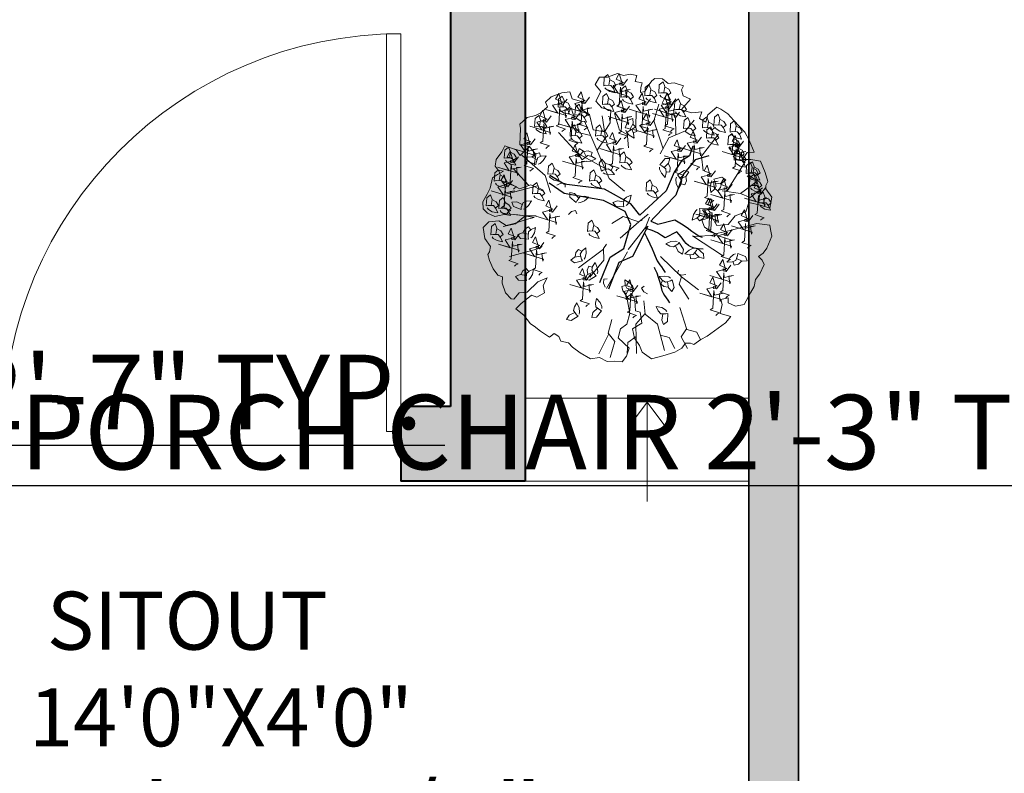
# Model space of a CAD drawing. Units: inches. Extents: x 2337 to 3570, y 1258 to 1938.
# Tile 7 of 30: x 2812 to 2931, y 1507 to 1598. Entities that reach past the tile are written whole.
import ezdxf

# ---------------------------------------------------------------- set-up
doc = ezdxf.new("R2010")
doc.units = ezdxf.units.IN
for name, color, linetype, lineweight in [('A-ANNO-DIMS', 2, 'Continuous', 18), ('A-ANNO-SYMB', 7, 'Continuous', 18), ('A-AREA-IDEN', 7, 'Continuous', 18), ('A-DOOR', 4, 'Continuous', 20), ('A-FLOR-STRS', 7, 'Continuous', 20), ('A-WALL', 7, 'Continuous', 40), ('ARBOL', 74, 'Continuous', 13), ('C-PROP', 7, 'Continuous', 35)]:
    doc.layers.add(name, color=color, linetype=linetype, lineweight=lineweight)
doc.layers.add('A-WALL-PATT', color=18, linetype='Continuous', lineweight=13, true_color=0x000000)
doc.layers.add('C-PROP-PATT', color=251, linetype='Continuous', lineweight=13, true_color=0x636466)
doc.layers.add('TALLO', color=36, linetype='Continuous')
doc.styles.get("Standard").update_dxf_attribs({"font": 'arial.ttf'})
doc.dimstyles.new('ISO-25', dxfattribs={"dimtxt": 9, "dimasz": 2.5, "dimexe": 1.25, "dimexo": 0.625, "dimtad": 1, "dimdec": 1, "dimlunit": 3, "dimtxsty": 'Standard', "dimcen": 2.5, "dimadec": 0, "dimazin": 0, "dimtfac": 1, "dimtdec": 1, "dimtmove": 0, "dimatfit": 3, "dimfxl": 1, "dimarcsym": 0})

# ---------------------------------------------------------------- blocks, each defined once
blk = doc.blocks.new('fresno')
at = {"layer": 'ARBOL'}
for p, q in [((2.96, 0.991), (3.575, 1.984)), ((-3.638, 1.194), (-4.164, 1.76)), ((-1.151, -0.932), (-1.99, -1.556)), ((-0.974, -3.757), (-1.31, -4.423))]:
    blk.add_line(p, q, dxfattribs=at)
blk.add_lwpolyline([(0.823, 4.745), (0.566, 4.764), (0.459, 4.687), (0.336, 4.518), (0.233, 4.322), (0.087, 4.298), (0.091, 4.464), (0.14, 4.621), (-0.09, 4.659), (-0.033, 4.863), (-0.264, 4.901), (-0.483, 4.866), (-0.686, 4.924), (-1.021, 4.801), (-1.288, 4.8), (-1.431, 4.563), (-1.234, 4.327), (-1.406, 4), (-1.205, 3.778), (-0.909, 3.705), (-0.931, 3.283), (-1.122, 2.983), (-1.491, 3.043), (-1.619, 3.562), (-1.9, 3.727), (-1.851, 3.982), (-2.197, 4.084), (-2.278, 4.31), (-2.543, 4.283), (-2.896, 4.152), (-3.091, 3.971), (-3.022, 3.817), (-3.244, 3.617), (-3.424, 3.528), (-3.697, 3.455), (-3.946, 3.236), (-3.922, 3.09), (-3.94, 2.548), (-3.617, 2.495), (-3.927, 2.19), (-4.062, 2.379), (-4.443, 2.512), (-4.546, 2.316), (-4.73, 2.062), (-4.767, 1.832), (-4.671, 1.698), (-4.486, 1.667), (-4.693, 1.559), (-4.854, 1.444), (-4.934, 1.102), (-5.037, 0.905), (-5.175, 0.644), (-5.166, 0.406), (-5.024, 0.264), (-4.781, 0.153), (-4.363, 0.249), (-4.014, 0.215), (-3.783, 0.177), (-3.46, 0.124), (-3.733, 0.051), (-4.132, -0.073), (-4.404, -0.146), (-4.639, 0.011), (-4.977, -0.028), (-5.172, -0.209), (-5.113, -0.574), (-4.921, -0.843), (-4.951, -1.027), (-5.012, -1.112), (-4.95, -1.311), (-4.83, -1.592), (-4.676, -1.807), (-4.518, -1.856), (-4.529, -2.068), (-4.417, -2.394), (-4.236, -2.59), (-4.143, -2.605), (-3.967, -2.397), (-3.703, -2.37), (-3.339, -2.027), (-3.032, -1.889), (-3.169, -2.15), (-3.115, -2.396), (-3.376, -2.542), (-3.552, -2.466), (-3.909, -2.762), (-4.077, -2.924), (-3.804, -3.135), (-3.592, -3.43), (-3.461, -3.499), (-3.253, -3.676), (-2.953, -3.867), (-2.792, -3.752), (-2.642, -3.848), (-2.572, -4.001), (-2.323, -4.066), (-2.18, -4.208), (-1.926, -4.392), (-1.58, -4.591), (-1.288, -4.545), (-1.027, -4.683), (-0.788, -4.675), (-0.531, -4.693), (-0.382, -4.505), (-0.29, -4.236), (-0.66, -3.891), (-0.588, -3.595), (-0.374, -3.441), (-0.267, -3.079), (-0.368, -2.541), (-0.208, -2.426), (-0.099, -2.633), (-0.087, -2.991), (0.071, -3.04), (0.129, -3.405), (-0.185, -3.59), (-0.119, -3.909), (0.055, -4.151), (0.136, -4.377), (0.456, -4.596), (0.828, -4.491), (1.227, -4.368), (1.461, -4.241), (1.583, -4.071), (1.748, -4.075), (1.86, -4.117), (2.101, -3.944), (2.308, -3.836), (2.925, -3.393), (3.101, -3.185), (2.74, -3.078), (2.812, -2.782), (2.769, -2.61), (3.015, -2.555), (3.012, -2.721), (3.254, -2.832), (3.546, -2.785), (3.752, -2.393), (3.882, -2.177), (3.92, -1.947), (4.069, -1.758), (4.214, -1.451), (4.144, -1.297), (4.021, -1.182), (4.182, -1.067), (4.304, -0.897), (4.464, -0.497), (4.429, -0.279), (4.406, -0.133), (3.964, -0.083), (3.074, -0.315), (2.582, -0.424), (2.217, -0.197), (2.136, 0.029), (2.462, 0.141), (2.628, -0.147), (3.012, -0.116), (3.249, 0.177), (3.602, 0.308), (3.701, 0.623), (4.089, 0.535), (4.404, 0.436), (4.464, 0.805), (4.272, 1.074), (4.267, 1.193), (4.336, 1.324), (4.243, 1.623), (4.092, 2.003), (3.769, 2.057), (3.485, 2.056), (3.642, 2.291), (3.88, 2.299), (3.71, 2.706), (3.563, 2.967), (3.201, 3.358), (3.001, 3.581), (2.766, 3.738), (2.635, 3.807), (2.332, 3.549), (2.268, 3.299), (2.052, 3.429), (2.136, 3.652), (1.798, 3.613), (1.437, 3.72), (1.755, 4.071), (1.513, 4.182), (1.451, 4.381), (1.519, 4.512), (1.204, 4.611), (1.012, 4.596)], close=True, dxfattribs=at)
for points in [[(-1.104, 4.45), (-1.063, 4.399), (-0.939, 4.325), (-0.757, 4.285), (-0.82, 4.431), (-0.903, 4.527), (-1.075, 4.533), (-1.143, 4.521), (-1.126, 4.792), (-1.002, 4.891), (-0.939, 4.738), (-0.975, 4.535)], [(-0.346, 4.735), (-0.501, 4.528), (-0.605, 4.545), (-0.605, 4.614), (-0.519, 4.563), (-0.622, 4.925), (-0.726, 4.735), (-0.484, 4.632), (-0.622, 4.58), (-0.829, 4.528), (-0.657, 4.27), (-1.053, 4.39), (-0.363, 4.183), (-0.381, 4.114), (-0.415, 4.373), (-0.26, 4.39), (-0.57, 4.321), (-0.588, 4.476), (-0.622, 3.89), (-0.708, 3.839), (-0.398, 3.735), (-0.467, 3.701), (-0.519, 3.649)], [(-0.935, 4.717), (-0.809, 4.65), (-0.736, 4.529), (-0.824, 4.459)], [(0.734, 4.203), (0.775, 4.152), (0.9, 4.078), (1.082, 4.038), (1.018, 4.185), (0.936, 4.281), (0.763, 4.287), (0.696, 4.274), (0.712, 4.546), (0.837, 4.645), (0.899, 4.491), (0.863, 4.289)], [(-1.623, 4.132), (-1.778, 3.925), (-1.882, 3.942), (-1.882, 4.011), (-1.795, 3.959), (-1.899, 4.321), (-2.002, 4.132), (-1.761, 4.028), (-1.899, 3.977), (-2.106, 3.925), (-1.933, 3.666), (-2.33, 3.787), (-1.64, 3.58), (-1.657, 3.511), (-1.692, 3.77), (-1.537, 3.787), (-1.847, 3.718), (-1.864, 3.873), (-1.899, 3.287), (-1.985, 3.235), (-1.675, 3.132), (-1.744, 3.097), (-1.795, 3.046)], [(-0.521, 4.069), (-0.48, 4.018), (-0.356, 3.944), (-0.174, 3.904), (-0.237, 4.051), (-0.32, 4.146), (-0.492, 4.152), (-0.56, 4.14), (-0.543, 4.411), (-0.419, 4.511), (-0.356, 4.357), (-0.392, 4.154)], [(-0.352, 4.337), (-0.226, 4.269), (-0.153, 4.148), (-0.241, 4.078)], [(0.263, 4.114), (0.304, 4.063), (0.429, 3.989), (0.611, 3.948), (0.547, 4.095), (0.465, 4.191), (0.293, 4.197), (0.225, 4.185), (0.242, 4.456), (0.366, 4.555), (0.428, 4.402), (0.393, 4.199)], [(0.433, 4.381), (0.558, 4.314), (0.631, 4.193), (0.544, 4.122)], [(0.904, 4.471), (1.029, 4.404), (1.102, 4.282), (1.015, 4.212)], [(-2.368, 4.073), (-2.523, 3.866), (-2.627, 3.883), (-2.627, 3.952), (-2.541, 3.9), (-2.644, 4.262), (-2.748, 4.073), (-2.506, 3.969), (-2.644, 3.918), (-2.851, 3.866), (-2.679, 3.607), (-3.075, 3.728), (-2.385, 3.521), (-2.403, 3.452), (-2.437, 3.711), (-2.282, 3.728), (-2.592, 3.659), (-2.61, 3.814), (-2.644, 3.228), (-2.73, 3.176), (-2.42, 3.073), (-2.489, 3.038), (-2.541, 2.987)], [(-2.629, 3.733), (-2.588, 3.682), (-2.463, 3.608), (-2.281, 3.568), (-2.345, 3.715), (-2.427, 3.81), (-2.6, 3.816), (-2.667, 3.804), (-2.651, 4.075), (-2.526, 4.175), (-2.464, 4.021), (-2.5, 3.818)], [(-2.459, 4), (-2.334, 3.933), (-2.261, 3.812), (-2.348, 3.742)], [(-1.149, 3.822), (-1.108, 3.771), (-0.983, 3.697), (-0.802, 3.657), (-0.865, 3.804), (-0.948, 3.9), (-1.12, 3.906), (-1.188, 3.893), (-1.171, 4.165), (-1.047, 4.264), (-0.984, 4.111), (-1.02, 3.908)], [(-0.287, 3.833), (-0.442, 3.626), (-0.546, 3.643), (-0.546, 3.712), (-0.46, 3.661), (-0.563, 4.023), (-0.667, 3.833), (-0.425, 3.73), (-0.563, 3.678), (-0.77, 3.626), (-0.598, 3.367), (-0.995, 3.488), (-0.304, 3.281), (-0.322, 3.212), (-0.356, 3.471), (-0.201, 3.488), (-0.511, 3.419), (-0.529, 3.574), (-0.563, 2.988), (-0.649, 2.936), (-0.339, 2.833), (-0.408, 2.799), (-0.46, 2.747)], [(-0.98, 4.09), (-0.854, 4.023), (-0.781, 3.901), (-0.869, 3.831)], [(0.413, 4.08), (0.258, 3.873), (0.154, 3.89), (0.154, 3.959), (0.241, 3.908), (0.137, 4.27), (0.034, 4.08), (0.275, 3.977), (0.137, 3.925), (-0.07, 3.873), (0.103, 3.614), (-0.294, 3.735), (0.396, 3.528), (0.379, 3.459), (0.344, 3.718), (0.499, 3.735), (0.189, 3.666), (0.172, 3.821), (0.137, 3.235), (0.051, 3.183), (0.361, 3.08), (0.292, 3.046), (0.241, 2.994)], [(1.189, 3.942), (1.034, 3.735), (0.931, 3.752), (0.931, 3.821), (1.017, 3.77), (0.913, 4.132), (0.81, 3.942), (1.051, 3.839), (0.913, 3.787), (0.706, 3.735), (0.879, 3.477), (0.482, 3.597), (1.172, 3.39), (1.155, 3.321), (1.12, 3.58), (1.276, 3.597), (0.965, 3.528), (0.948, 3.683), (0.913, 3.097), (0.827, 3.046), (1.138, 2.942), (1.069, 2.908), (1.017, 2.856)], [(1.259, 4.08), (1.103, 3.873), (1, 3.89), (1, 3.959), (1.086, 3.908), (0.982, 4.27), (0.879, 4.08), (1.12, 3.977), (0.982, 3.925), (0.775, 3.873), (0.948, 3.614), (0.551, 3.735), (1.241, 3.528), (1.224, 3.459), (1.189, 3.718), (1.345, 3.735), (1.034, 3.666), (1.017, 3.821), (0.982, 3.235), (0.896, 3.183), (1.207, 3.08), (1.138, 3.046), (1.086, 2.994)], [(1.25, 3.643), (1.291, 3.592), (1.416, 3.518), (1.597, 3.478), (1.534, 3.625), (1.451, 3.721), (1.279, 3.727), (1.211, 3.714), (1.228, 3.985), (1.352, 4.085), (1.415, 3.931), (1.379, 3.729)], [(-2.898, 3.511), (-3.053, 3.304), (-3.157, 3.321), (-3.157, 3.39), (-3.071, 3.339), (-3.174, 3.701), (-3.278, 3.511), (-3.036, 3.408), (-3.174, 3.356), (-3.381, 3.304), (-3.209, 3.046), (-3.605, 3.166), (-2.915, 2.959), (-2.932, 2.89), (-2.967, 3.149), (-2.812, 3.166), (-3.122, 3.097), (-3.14, 3.253), (-3.174, 2.666), (-3.26, 2.615), (-2.95, 2.511), (-3.019, 2.477), (-3.071, 2.425)], [(-1.951, 3.597), (-2.106, 3.39), (-2.209, 3.408), (-2.209, 3.477), (-2.123, 3.425), (-2.227, 3.787), (-2.33, 3.597), (-2.089, 3.494), (-2.227, 3.442), (-2.434, 3.39), (-2.261, 3.132), (-2.658, 3.252), (-1.968, 3.046), (-1.985, 2.977), (-2.02, 3.235), (-1.864, 3.252), (-2.175, 3.183), (-2.192, 3.339), (-2.227, 2.752), (-2.313, 2.701), (-2.002, 2.597), (-2.071, 2.563), (-2.123, 2.511)], [(-2.068, 3.464), (-2.027, 3.413), (-1.903, 3.339), (-1.721, 3.299), (-1.784, 3.446), (-1.867, 3.542), (-2.039, 3.547), (-2.107, 3.535), (-2.09, 3.806), (-1.966, 3.906), (-1.903, 3.752), (-1.939, 3.55)], [(-1.899, 3.732), (-1.773, 3.664), (-1.7, 3.543), (-1.788, 3.473)], [(-0.063, 3.671), (-0.069, 3.151), (-0.364, 2.965), (-0.319, 2.449)], [(0.837, 2.414), (0.533, 3.352), (0.697, 3.906)], [(1.259, 2.882), (1.254, 3.446), (1.381, 3.636)], [(1.419, 3.911), (1.545, 3.844), (1.618, 3.722), (1.53, 3.652)], [(-3.413, 3.083), (-3.373, 3.032), (-3.248, 2.958), (-3.066, 2.918), (-3.129, 3.065), (-3.212, 3.161), (-3.384, 3.167), (-3.452, 3.154), (-3.435, 3.425), (-3.311, 3.525), (-3.248, 3.371), (-3.284, 3.169)], [(-3.244, 3.351), (-3.118, 3.284), (-3.045, 3.162), (-3.133, 3.092)], [(-0.448, 1), (-0.961, 1.419), (-1.784, 3.341)], [(-1.367, 2.367), (-1.081, 2.78), (-1.193, 3.514)], [(-0.923, 3.449), (-0.951, 3.425), (-0.93, 3.313)], [(-0.358, 2.895), (-0.615, 3.037), (-0.783, 3.596)], [(-0.41, 3.035), (-0.387, 2.974), (-0.291, 2.865), (-0.131, 2.771), (-0.146, 2.93), (-0.195, 3.047), (-0.357, 3.106), (-0.425, 3.115), (-0.325, 3.368), (-0.176, 3.424), (-0.164, 3.258), (-0.261, 3.077)], [(0.558, 3.402), (0.403, 3.195), (0.299, 3.212), (0.299, 3.281), (0.386, 3.23), (0.282, 3.592), (0.179, 3.402), (0.42, 3.299), (0.282, 3.247), (0.075, 3.195), (0.248, 2.936), (-0.149, 3.057), (0.541, 2.85), (0.524, 2.781), (0.489, 3.04), (0.644, 3.057), (0.334, 2.988), (0.317, 3.143), (0.282, 2.557), (0.196, 2.505), (0.506, 2.402), (0.437, 2.368), (0.386, 2.316)], [(0.746, 2.242), (1.034, 2.786), (1.584, 3.019), (1.879, 3.374)], [(1.564, 3.016), (1.605, 2.965), (1.729, 2.891), (1.911, 2.851), (1.848, 2.998), (1.765, 3.094), (1.593, 3.099), (1.525, 3.087), (1.542, 3.358), (1.666, 3.458), (1.729, 3.304), (1.693, 3.102)], [(2.191, 3.038), (2.232, 2.987), (2.357, 2.913), (2.539, 2.873), (2.475, 3.02), (2.393, 3.116), (2.221, 3.122), (2.153, 3.109), (2.17, 3.381), (2.294, 3.48), (2.356, 3.326), (2.321, 3.124)], [(2.361, 3.306), (2.486, 3.239), (2.559, 3.117), (2.472, 3.047)], [(2.573, 3.128), (2.613, 3.077), (2.738, 3.003), (2.92, 2.963), (2.857, 3.11), (2.774, 3.205), (2.602, 3.211), (2.534, 3.199), (2.551, 3.47), (2.675, 3.57), (2.738, 3.416), (2.702, 3.214)], [(2.742, 3.396), (2.868, 3.328), (2.941, 3.207), (2.853, 3.137)], [(3.111, 2.904), (3.152, 2.853), (3.276, 2.779), (3.458, 2.739), (3.395, 2.886), (3.312, 2.981), (3.14, 2.987), (3.072, 2.975), (3.089, 3.246), (3.213, 3.346), (3.276, 3.192), (3.24, 2.99)], [(-2.225, 2.77), (-2.184, 2.718), (-2.06, 2.645), (-1.878, 2.604), (-1.941, 2.751), (-2.024, 2.847), (-2.196, 2.853), (-2.264, 2.84), (-2.247, 3.112), (-2.123, 3.211), (-2.06, 3.058), (-2.096, 2.855)], [(-1.575, 2.854), (-2.052, 2.969), (-2.2, 3.178)], [(-2.056, 3.037), (-1.93, 2.97), (-1.857, 2.849), (-1.945, 2.778)], [(-1.373, 2.77), (-1.332, 2.718), (-1.208, 2.645), (-1.026, 2.604), (-1.089, 2.751), (-1.172, 2.847), (-1.344, 2.853), (-1.412, 2.84), (-1.395, 3.112), (-1.271, 3.211), (-1.208, 3.058), (-1.244, 2.855)], [(-0.57, 2.77), (-0.726, 2.563), (-0.829, 2.58), (-0.829, 2.649), (-0.743, 2.597), (-0.846, 2.959), (-0.95, 2.77), (-0.708, 2.666), (-0.846, 2.615), (-1.053, 2.563), (-0.881, 2.304), (-1.278, 2.425), (-0.588, 2.218), (-0.605, 2.149), (-0.639, 2.408), (-0.484, 2.425), (-0.795, 2.356), (-0.812, 2.511), (-0.846, 1.925), (-0.933, 1.873), (-0.622, 1.77), (-0.691, 1.735), (-0.743, 1.684)], [(-1.204, 3.037), (-1.078, 2.97), (-1.005, 2.849), (-1.093, 2.778)], [(-0.166, 3.238), (-0.068, 3.135), (-0.036, 2.997), (-0.141, 2.957)], [(2.121, 2.804), (1.966, 2.597), (1.862, 2.615), (1.862, 2.683), (1.949, 2.632), (1.845, 2.994), (1.742, 2.804), (1.983, 2.701), (1.845, 2.649), (1.638, 2.597), (1.811, 2.339), (1.414, 2.459), (2.104, 2.252), (2.087, 2.184), (2.052, 2.442), (2.207, 2.459), (1.897, 2.39), (1.88, 2.546), (1.845, 1.959), (1.759, 1.908), (2.069, 1.804), (2, 1.77), (1.949, 1.718)], [(1.733, 3.284), (1.859, 3.216), (1.932, 3.095), (1.844, 3.025)], [(2.326, 2.702), (2.367, 2.651), (2.492, 2.577), (2.673, 2.537), (2.61, 2.684), (2.527, 2.78), (2.355, 2.786), (2.287, 2.773), (2.304, 3.045), (2.428, 3.144), (2.491, 2.99), (2.455, 2.788)], [(2.495, 2.97), (2.621, 2.903), (2.694, 2.781), (2.606, 2.711)], [(3.28, 3.172), (3.406, 3.104), (3.479, 2.983), (3.391, 2.913)], [(-3.434, 2.752), (-3.59, 2.546), (-3.693, 2.563), (-3.693, 2.632), (-3.607, 2.58), (-3.71, 2.942), (-3.814, 2.752), (-3.572, 2.649), (-3.71, 2.597), (-3.917, 2.546), (-3.745, 2.287), (-4.142, 2.408), (-3.452, 2.201), (-3.469, 2.132), (-3.503, 2.39), (-3.348, 2.408), (-3.659, 2.339), (-3.676, 2.494), (-3.71, 1.908), (-3.797, 1.856), (-3.486, 1.753), (-3.555, 1.718), (-3.607, 1.666)], [(-1.112, 1.773), (-2.014, 2.265), (-2.654, 2.957)], [(1.586, 2.528), (1.431, 2.321), (1.327, 2.339), (1.327, 2.408), (1.414, 2.356), (1.31, 2.718), (1.207, 2.528), (1.448, 2.425), (1.31, 2.373), (1.103, 2.321), (1.276, 2.063), (0.879, 2.184), (1.569, 1.977), (1.552, 1.908), (1.517, 2.166), (1.673, 2.184), (1.362, 2.115), (1.345, 2.27), (1.31, 1.684), (1.224, 1.632), (1.535, 1.528), (1.466, 1.494), (1.414, 1.442)], [(2.171, 1.674), (2.121, 2.172), (2.689, 2.898)], [(3.519, 2.666), (3.363, 2.459), (3.26, 2.477), (3.26, 2.546), (3.346, 2.494), (3.243, 2.856), (3.139, 2.666), (3.381, 2.563), (3.243, 2.511), (3.036, 2.459), (3.208, 2.201), (2.811, 2.321), (3.501, 2.115), (3.484, 2.046), (3.45, 2.304), (3.605, 2.321), (3.294, 2.252), (3.277, 2.408), (3.243, 1.821), (3.156, 1.77), (3.467, 1.666), (3.398, 1.632), (3.346, 1.58)], [(3.043, 2.478), (3.084, 2.427), (3.209, 2.353), (3.391, 2.313), (3.327, 2.46), (3.245, 2.556), (3.073, 2.562), (3.005, 2.549), (3.022, 2.82), (3.146, 2.92), (3.208, 2.766), (3.173, 2.564)], [(3.213, 2.746), (3.338, 2.679), (3.411, 2.557), (3.324, 2.487)], [(-3.986, 2.149), (-4.142, 1.942), (-4.245, 1.959), (-4.245, 2.028), (-4.159, 1.977), (-4.262, 2.339), (-4.366, 2.149), (-4.124, 2.046), (-4.262, 1.994), (-4.47, 1.942), (-4.297, 1.684), (-4.694, 1.804), (-4.004, 1.597), (-4.021, 1.528), (-4.055, 1.787), (-3.9, 1.804), (-4.211, 1.735), (-4.228, 1.89), (-4.262, 1.304), (-4.349, 1.253), (-4.038, 1.149), (-4.107, 1.115), (-4.159, 1.063)], [(-4.422, 2.03), (-4.381, 1.979), (-4.257, 1.905), (-4.075, 1.865), (-4.138, 2.012), (-4.221, 2.108), (-4.393, 2.114), (-4.461, 2.101), (-4.444, 2.372), (-4.32, 2.472), (-4.257, 2.318), (-4.293, 2.116)], [(-3.468, 1.85), (-3.409, 2.222), (-3.628, 2.505)], [(-1.817, 2.351), (-1.972, 2.144), (-2.075, 2.162), (-2.075, 2.231), (-1.989, 2.179), (-2.093, 2.541), (-2.196, 2.351), (-1.955, 2.248), (-2.093, 2.196), (-2.3, 2.144), (-2.127, 1.886), (-2.524, 2.006), (-1.834, 1.8), (-1.851, 1.731), (-1.886, 1.989), (-1.73, 2.006), (-2.041, 1.937), (-2.058, 2.093), (-2.093, 1.506), (-2.179, 1.455), (-1.868, 1.351), (-1.937, 1.317), (-1.989, 1.265)], [(-1.786, 2.007), (-1.722, 1.99), (-1.578, 2.003), (-1.407, 2.078), (-1.545, 2.159), (-1.668, 2.188), (-1.811, 2.092), (-1.859, 2.042), (-2.004, 2.271), (-1.962, 2.425), (-1.821, 2.337), (-1.731, 2.152)], [(-1.806, 2.323), (-1.665, 2.343), (-1.534, 2.287), (-1.564, 2.179)], [(-0.566, 1.873), (-0.525, 1.822), (-0.4, 1.748), (-0.219, 1.708), (-0.282, 1.855), (-0.365, 1.951), (-0.537, 1.957), (-0.605, 1.944), (-0.588, 2.216), (-0.464, 2.315), (-0.401, 2.162), (-0.437, 1.959)], [(3.178, 2.165), (3.219, 2.113), (3.344, 2.04), (3.525, 1.999), (3.462, 2.146), (3.379, 2.242), (3.207, 2.248), (3.139, 2.236), (3.156, 2.507), (3.28, 2.606), (3.343, 2.453), (3.307, 2.25)], [(3.245, 1.963), (3.286, 1.912), (3.411, 1.838), (3.593, 1.798), (3.529, 1.945), (3.447, 2.041), (3.274, 2.046), (3.206, 2.034), (3.223, 2.305), (3.347, 2.405), (3.41, 2.251), (3.374, 2.049)], [(3.347, 2.432), (3.473, 2.365), (3.546, 2.244), (3.458, 2.173)], [(-4.253, 2.298), (-4.127, 2.231), (-4.054, 2.109), (-4.142, 2.039)], [(-2.916, 0.958), (-3.096, 1.528), (-3.871, 2.197)], [(-3.331, 1.905), (-3.269, 1.928), (-3.161, 2.024), (-3.066, 2.184), (-3.226, 2.169), (-3.342, 2.121), (-3.401, 1.958), (-3.41, 1.89), (-3.663, 1.99), (-3.719, 2.139), (-3.554, 2.151), (-3.372, 2.054)], [(-3.533, 2.149), (-3.43, 2.247), (-3.292, 2.279), (-3.252, 2.174)], [(-1.164, 1.612), (-1.109, 1.576), (-0.967, 1.544), (-0.782, 1.562), (-0.888, 1.682), (-0.996, 1.748), (-1.162, 1.7), (-1.222, 1.667), (-1.29, 1.93), (-1.203, 2.063), (-1.096, 1.937), (-1.067, 1.733)], [(-0.397, 2.141), (-0.271, 2.074), (-0.198, 1.952), (-0.286, 1.882)], [(0.72, 1.798), (0.723, 1.733), (0.781, 1.6), (0.904, 1.46), (0.939, 1.616), (0.929, 1.742), (0.793, 1.848), (0.73, 1.878), (0.904, 2.088), (1.062, 2.095), (1.023, 1.934), (0.875, 1.791)], [(3.415, 2.231), (3.54, 2.163), (3.613, 2.042), (3.525, 1.972)], [(3.716, 1.537), (3.757, 1.486), (3.882, 1.412), (4.063, 1.372), (4, 1.519), (3.917, 1.615), (3.745, 1.621), (3.677, 1.608), (3.694, 1.88), (3.818, 1.979), (3.881, 1.825), (3.845, 1.623)], [(-4.759, 1.269), (-4.718, 1.217), (-4.593, 1.144), (-4.411, 1.103), (-4.475, 1.25), (-4.557, 1.346), (-4.729, 1.352), (-4.797, 1.339), (-4.78, 1.611), (-4.656, 1.71), (-4.594, 1.557), (-4.629, 1.354)], [(-2.965, 1.493), (-2.924, 1.441), (-2.799, 1.368), (-2.618, 1.327), (-2.681, 1.474), (-2.764, 1.57), (-2.936, 1.576), (-3.004, 1.564), (-2.987, 1.835), (-2.863, 1.934), (-2.8, 1.781), (-2.836, 1.578)], [(-2.796, 1.76), (-2.67, 1.693), (-2.597, 1.572), (-2.685, 1.501)], [(-1.575, 1.269), (-1.534, 1.217), (-1.409, 1.144), (-1.228, 1.103), (-1.291, 1.25), (-1.373, 1.346), (-1.546, 1.352), (-1.614, 1.339), (-1.597, 1.611), (-1.473, 1.71), (-1.41, 1.557), (-1.446, 1.354)], [(-1.085, 1.919), (-0.945, 1.893), (-0.838, 1.801), (-0.9, 1.707)], [(1.014, 1.915), (1.077, 1.787), (1.064, 1.646), (0.952, 1.64)], [(1.283, 1.469), (1.266, 1.405), (1.279, 1.261), (1.354, 1.09), (1.435, 1.228), (1.464, 1.351), (1.368, 1.494), (1.318, 1.542), (1.547, 1.687), (1.7, 1.645), (1.613, 1.504), (1.428, 1.414)], [(2.587, 1.684), (2.432, 1.477), (2.328, 1.494), (2.328, 1.563), (2.414, 1.511), (2.311, 1.873), (2.207, 1.684), (2.449, 1.58), (2.311, 1.528), (2.104, 1.477), (2.276, 1.218), (1.88, 1.339), (2.57, 1.132), (2.552, 1.063), (2.518, 1.321), (2.673, 1.339), (2.363, 1.27), (2.345, 1.425), (2.311, 0.839), (2.225, 0.787), (2.535, 0.684), (2.466, 0.649), (2.414, 0.597)], [(3.649, 1.515), (3.69, 1.464), (3.814, 1.39), (3.996, 1.35), (3.933, 1.497), (3.85, 1.592), (3.678, 1.598), (3.61, 1.586), (3.627, 1.857), (3.751, 1.957), (3.814, 1.803), (3.778, 1.601)], [(3.818, 1.783), (3.944, 1.715), (4.017, 1.594), (3.929, 1.524)], [(3.885, 1.805), (4.011, 1.738), (4.084, 1.616), (3.996, 1.546)], [(-4.193, 1.356), (-4.349, 1.149), (-4.452, 1.166), (-4.452, 1.235), (-4.366, 1.184), (-4.469, 1.546), (-4.573, 1.356), (-4.331, 1.253), (-4.469, 1.201), (-4.677, 1.149), (-4.504, 0.89), (-4.901, 1.011), (-4.211, 0.804), (-4.228, 0.735), (-4.262, 0.994), (-4.107, 1.011), (-4.418, 0.942), (-4.435, 1.097), (-4.469, 0.511), (-4.556, 0.459), (-4.245, 0.356), (-4.314, 0.322), (-4.366, 0.27)], [(-4.589, 1.536), (-4.464, 1.469), (-4.391, 1.348), (-4.478, 1.277)], [(-3.192, 1.017), (-3.578, 1.215), (-3.949, 1.081), (-4.398, 1.339)], [(-1.406, 1.536), (-1.28, 1.469), (-1.207, 1.348), (-1.295, 1.277)], [(0.308, 0.933), (0.349, 0.881), (0.474, 0.807), (0.656, 0.767), (0.592, 0.914), (0.51, 1.01), (0.337, 1.016), (0.27, 1.003), (0.286, 1.275), (0.411, 1.374), (0.473, 1.221), (0.437, 1.018)], [(1.599, 1.489), (1.618, 1.348), (1.563, 1.217), (1.455, 1.247)], [(2.479, 1.34), (2.443, 1.285), (2.411, 1.143), (2.429, 0.958), (2.549, 1.064), (2.615, 1.172), (2.567, 1.338), (2.534, 1.398), (2.797, 1.466), (2.93, 1.379), (2.804, 1.272), (2.6, 1.243)], [(3.139, 1.235), (2.984, 1.028), (2.88, 1.046), (2.88, 1.115), (2.967, 1.063), (2.863, 1.425), (2.759, 1.235), (3.001, 1.132), (2.863, 1.08), (2.656, 1.028), (2.828, 0.77), (2.432, 0.891), (3.122, 0.684), (3.105, 0.615), (3.07, 0.873), (3.225, 0.891), (2.915, 0.822), (2.897, 0.977), (2.863, 0.391), (2.777, 0.339), (3.087, 0.235), (3.018, 0.201), (2.967, 0.149)], [(4.01, 1.36), (3.422, 0.918)], [(3.761, 1.112), (3.802, 1.061), (3.926, 0.987), (4.108, 0.947), (4.045, 1.093), (3.962, 1.189), (3.79, 1.195), (3.722, 1.183), (3.739, 1.454), (3.863, 1.553), (3.926, 1.4), (3.89, 1.197)], [(3.93, 1.379), (4.056, 1.312), (4.129, 1.191), (4.041, 1.121)], [(-3.354, 1.176), (-4.529, 0.864)], [(-3.481, 0.843), (-3.44, 0.792), (-3.315, 0.718), (-3.133, 0.678), (-3.197, 0.825), (-3.279, 0.92), (-3.451, 0.926), (-3.519, 0.914), (-3.502, 1.185), (-3.378, 1.285), (-3.316, 1.131), (-3.351, 0.928)], [(-3.311, 1.111), (-3.186, 1.043), (-3.113, 0.922), (-3.2, 0.852)], [(-2.703, 1.201), (-2.575, 1.263), (-2.433, 1.251), (-2.428, 1.139)], [(0.478, 1.2), (0.603, 1.133), (0.676, 1.011), (0.589, 0.941)], [(2.786, 1.261), (2.76, 1.121), (2.668, 1.014), (2.574, 1.076)], [(2.808, 1.015), (3.422, 0.918), (3.422, 0.918), (3.748, 0.794), (4.154, 1.111)], [(4.26, 1.115), (4.105, 0.908), (4.002, 0.925), (4.002, 0.994), (4.088, 0.942), (3.984, 1.304), (3.881, 1.115), (4.122, 1.011), (3.984, 0.959), (3.777, 0.908), (3.95, 0.649), (3.553, 0.77), (4.243, 0.563), (4.226, 0.494), (4.191, 0.753), (4.347, 0.77), (4.036, 0.701), (4.019, 0.856), (3.984, 0.27), (3.898, 0.218), (4.209, 0.115), (4.14, 0.08), (4.088, 0.029)], [(-5.028, 0.44), (-4.987, 0.388), (-4.862, 0.315), (-4.68, 0.274), (-4.744, 0.421), (-4.826, 0.517), (-4.998, 0.523), (-5.066, 0.511), (-5.049, 0.782), (-4.925, 0.881), (-4.863, 0.728), (-4.898, 0.525)], [(-4.858, 0.707), (-4.733, 0.64), (-4.66, 0.519), (-4.747, 0.448)], [(-4.602, 0.35), (-4.561, 0.299), (-4.436, 0.225), (-4.254, 0.185), (-4.318, 0.332), (-4.4, 0.428), (-4.572, 0.433), (-4.64, 0.421), (-4.623, 0.692), (-4.499, 0.792), (-4.437, 0.638), (-4.472, 0.436)], [(-3.824, 0.404), (-3.763, 0.427), (-3.654, 0.523), (-3.559, 0.683), (-3.719, 0.668), (-3.835, 0.62), (-3.894, 0.457), (-3.903, 0.389), (-4.156, 0.489), (-4.212, 0.638), (-4.047, 0.65), (-3.865, 0.553)], [(-2.698, 0.509), (-2.854, 0.302), (-2.957, 0.319), (-2.957, 0.388), (-2.871, 0.336), (-2.974, 0.698), (-3.078, 0.509), (-2.836, 0.405), (-2.974, 0.353), (-3.182, 0.302), (-3.009, 0.043), (-3.406, 0.164), (-2.716, -0.043), (-2.733, -0.112), (-2.767, 0.147), (-2.612, 0.164), (-2.923, 0.095), (-2.94, 0.25), (-2.974, -0.336), (-3.061, -0.388), (-2.75, -0.491), (-2.819, -0.526), (-2.871, -0.577)], [(-1.981, 0.615), (-1.915, 0.618), (-1.782, 0.676), (-1.643, 0.799), (-1.799, 0.834), (-1.925, 0.824), (-2.031, 0.688), (-2.061, 0.626), (-2.27, 0.799), (-2.278, 0.958), (-2.117, 0.918), (-1.974, 0.77)], [(-0.397, 0.517), (-0.346, 0.557), (-0.272, 0.682), (-0.232, 0.864), (-0.379, 0.801), (-0.474, 0.718), (-0.48, 0.546), (-0.468, 0.478), (-0.739, 0.495), (-0.838, 0.619), (-0.685, 0.682), (-0.482, 0.646)], [(2.639, 0.58), (2.483, 0.373), (2.38, 0.391), (2.38, 0.46), (2.466, 0.408), (2.363, 0.77), (2.259, 0.58), (2.501, 0.477), (2.363, 0.425), (2.156, 0.373), (2.328, 0.115), (1.931, 0.235), (2.621, 0.029), (2.604, -0.04), (2.57, 0.218), (2.725, 0.235), (2.414, 0.166), (2.397, 0.322), (2.363, -0.265), (2.276, -0.316), (2.587, -0.42), (2.518, -0.454), (2.466, -0.506)], [(2.708, 0.563), (2.552, 0.356), (2.449, 0.373), (2.449, 0.442), (2.535, 0.391), (2.432, 0.753), (2.328, 0.563), (2.57, 0.46), (2.432, 0.408), (2.225, 0.356), (2.397, 0.097), (2, 0.218), (2.69, 0.011), (2.673, -0.058), (2.639, 0.201), (2.794, 0.218), (2.483, 0.149), (2.466, 0.304), (2.432, -0.282), (2.345, -0.334), (2.656, -0.437), (2.587, -0.471), (2.535, -0.523)], [(4.075, 0.529), (4.116, 0.478), (4.24, 0.404), (4.422, 0.364), (4.359, 0.511), (4.276, 0.607), (4.104, 0.613), (4.036, 0.6), (4.053, 0.871), (4.177, 0.971), (4.24, 0.817), (4.204, 0.615)], [(4.244, 0.797), (4.37, 0.73), (4.443, 0.608), (4.355, 0.538)], [(-4.432, 0.618), (-4.307, 0.55), (-4.234, 0.429), (-4.321, 0.359)], [(-2.322, 0.222), (-2.219, 0.321), (-2.081, 0.353), (-2.042, 0.248)], [(1.978, 0.384), (1.927, 0.343), (1.853, 0.218), (1.813, 0.036), (1.96, 0.1), (2.056, 0.182), (2.061, 0.355), (2.049, 0.422), (2.32, 0.406), (2.42, 0.281), (2.266, 0.219), (2.064, 0.254)], [(3.829, 0.184), (3.674, -0.023), (3.57, -0.006), (3.57, 0.063), (3.657, 0.011), (3.553, 0.373), (3.45, 0.184), (3.691, 0.08), (3.553, 0.029), (3.346, -0.023), (3.519, -0.282), (3.122, -0.161), (3.812, -0.368), (3.795, -0.437), (3.76, -0.178), (3.915, -0.161), (3.605, -0.23), (3.588, -0.075), (3.553, -0.661), (3.467, -0.713), (3.777, -0.816), (3.708, -0.851), (3.657, -0.902)], [(-3.394, 0.18), (-3.77, 0.182), (-4.532, 0.27)], [(-3.77, 0.182), (-4.09, -0.088), (-4.494, -0.18)], [(-1.642, -0.412), (-1.601, -0.463), (-1.477, -0.537), (-1.295, -0.577), (-1.358, -0.43), (-1.441, -0.334), (-1.613, -0.328), (-1.681, -0.341), (-1.664, -0.069), (-1.54, 0.03), (-1.477, -0.124), (-1.513, -0.326)], [(0.03, -0.026), (-0.491, 0.154), (-0.871, -0.08)], [(-0.596, -0.564), (0.03, -0.026), (0.339, 0.235)], [(0.38, 0.131), (0.248, -0.21), (-0.33, -0.951)], [(2.246, 0.214), (2.178, 0.089), (2.057, 0.016), (1.987, 0.103)], [(-4.871, -0.524), (-4.83, -0.575), (-4.705, -0.649), (-4.523, -0.689), (-4.587, -0.542), (-4.669, -0.446), (-4.841, -0.44), (-4.909, -0.453), (-4.893, -0.181), (-4.768, -0.082), (-4.706, -0.236), (-4.741, -0.438)], [(-4.701, -0.256), (-4.576, -0.323), (-4.503, -0.445), (-4.59, -0.515)], [(-3.952, -0.42), (-4.107, -0.627), (-4.211, -0.609), (-4.211, -0.54), (-4.124, -0.592), (-4.228, -0.23), (-4.331, -0.42), (-4.09, -0.523), (-4.228, -0.575), (-4.435, -0.627), (-4.262, -0.885), (-4.659, -0.765), (-3.969, -0.971), (-3.986, -1.04), (-4.021, -0.782), (-3.866, -0.765), (-4.176, -0.834), (-4.193, -0.678), (-4.228, -1.265), (-4.314, -1.316), (-4.004, -1.42), (-4.073, -1.454), (-4.124, -1.506)], [(-3.58, -0.559), (-3.529, -0.518), (-3.455, -0.393), (-3.415, -0.211), (-3.562, -0.275), (-3.658, -0.357), (-3.664, -0.53), (-3.651, -0.597), (-3.923, -0.581), (-4.022, -0.456), (-3.868, -0.394), (-3.666, -0.43)], [(-3.848, -0.389), (-3.781, -0.264), (-3.659, -0.191), (-3.589, -0.278)], [(-1.473, -0.144), (-1.347, -0.211), (-1.274, -0.333), (-1.362, -0.403)], [(3.139, -0.282), (2.984, -0.489), (2.88, -0.471), (2.88, -0.402), (2.967, -0.454), (2.863, -0.092), (2.759, -0.282), (3.001, -0.385), (2.863, -0.437), (2.656, -0.489), (2.828, -0.747), (2.432, -0.627), (3.122, -0.834), (3.105, -0.902), (3.07, -0.644), (3.225, -0.627), (2.915, -0.696), (2.897, -0.54), (2.863, -1.127), (2.777, -1.178), (3.087, -1.282), (3.018, -1.316), (2.967, -1.368)], [(-3.141, -0.713), (-3.296, -0.92), (-3.4, -0.902), (-3.4, -0.834), (-3.314, -0.885), (-3.417, -0.523), (-3.521, -0.713), (-3.279, -0.816), (-3.417, -0.868), (-3.624, -0.92), (-3.452, -1.178), (-3.848, -1.058), (-3.158, -1.265), (-3.175, -1.333), (-3.21, -1.075), (-3.055, -1.058), (-3.365, -1.127), (-3.383, -0.971), (-3.417, -1.558), (-3.503, -1.609), (-3.193, -1.713), (-3.262, -1.747), (-3.314, -1.799)], [(1.822, -0.495), (2.859, -1.165)], [(1.846, -0.51), (2.605, -0.469), (3.129, -0.637)], [(-3.195, -0.824), (-3.267, -0.898), (-4.285, -1.185)], [(-1.794, -1.268), (-1.758, -1.214), (-1.726, -1.072), (-1.744, -0.887), (-1.865, -0.993), (-1.93, -1.101), (-1.883, -1.266), (-1.85, -1.327), (-2.113, -1.395), (-2.246, -1.307), (-2.119, -1.2), (-1.916, -1.172)], [(-2.101, -1.19), (-2.076, -1.05), (-1.983, -0.943), (-1.889, -1.004)], [(-1.047, -0.767), (-1.151, -0.913), (-1.144, -1.307), (-1.61, -1.871)], [(1.304, -0.681), (1.241, -0.664), (1.097, -0.678), (0.926, -0.752), (1.064, -0.833), (1.187, -0.862), (1.33, -0.766), (1.377, -0.716), (1.523, -0.945), (1.481, -1.099), (1.34, -1.011), (1.25, -0.826)], [(1.903, -0.903), (1.837, -0.905), (1.704, -0.963), (1.565, -1.086), (1.721, -1.122), (1.847, -1.111), (1.953, -0.975), (1.983, -0.913), (2.192, -1.086), (2.2, -1.245), (2.039, -1.205), (1.896, -1.057)], [(-0.346, -1.024), (-1.05, -2.251)], [(0.748, -1.185), (1.452, -1.855), (2.021, -2.292)], [(2.02, -1.197), (1.891, -1.259), (1.75, -1.247), (1.745, -1.134)], [(3.105, -1.471), (2.949, -1.678), (2.846, -1.661), (2.846, -1.592), (2.932, -1.644), (2.829, -1.282), (2.725, -1.471), (2.967, -1.575), (2.829, -1.627), (2.621, -1.678), (2.794, -1.937), (2.397, -1.816), (3.087, -2.023), (3.07, -2.092), (3.036, -1.833), (3.191, -1.816), (2.88, -1.885), (2.863, -1.73), (2.829, -2.316), (2.742, -2.368), (3.053, -2.471), (2.984, -2.506), (2.932, -2.558)], [(3.253, -1.094), (3.192, -1.117), (3.083, -1.213), (2.988, -1.374), (3.148, -1.359), (3.264, -1.31), (3.323, -1.148), (3.332, -1.079), (3.585, -1.179), (3.641, -1.328), (3.476, -1.34), (3.294, -1.244)], [(-3.648, -1.948), (-3.596, -1.907), (-3.523, -1.782), (-3.482, -1.6), (-3.629, -1.664), (-3.725, -1.746), (-3.731, -1.919), (-3.719, -1.986), (-3.99, -1.97), (-4.089, -1.845), (-3.936, -1.783), (-3.733, -1.819)], [(-3.915, -1.778), (-3.848, -1.653), (-3.727, -1.58), (-3.656, -1.667)], [(-1.571, -1.764), (-1.726, -1.971), (-1.83, -1.954), (-1.83, -1.885), (-1.744, -1.937), (-1.847, -1.575), (-1.951, -1.764), (-1.709, -1.868), (-1.847, -1.92), (-2.054, -1.971), (-1.882, -2.23), (-2.278, -2.109), (-1.588, -2.316), (-1.605, -2.385), (-1.64, -2.127), (-1.485, -2.109), (-1.795, -2.178), (-1.813, -2.023), (-1.847, -2.609), (-1.933, -2.661), (-1.623, -2.764), (-1.692, -2.799), (-1.744, -2.851)], [(-1.361, -1.756), (-1.343, -1.693), (-1.357, -1.548), (-1.431, -1.377), (-1.513, -1.515), (-1.542, -1.638), (-1.445, -1.781), (-1.395, -1.829), (-1.625, -1.974), (-1.778, -1.932), (-1.691, -1.791), (-1.506, -1.701)], [(-1.677, -1.776), (-1.696, -1.635), (-1.641, -1.504), (-1.533, -1.534)], [(1.593, -1.781), (1.452, -1.801), (1.322, -1.746), (1.352, -1.637)], [(3.455, -1.338), (3.352, -1.437), (3.214, -1.469), (3.175, -1.364)], [(-1.092, -2.202), (-1.154, -2.074), (-1.142, -1.933), (-1.03, -1.928)], [(-0.001, -2.144), (-0.156, -2.351), (-0.26, -2.333), (-0.26, -2.264), (-0.174, -2.316), (-0.277, -1.954), (-0.381, -2.144), (-0.139, -2.247), (-0.277, -2.299), (-0.484, -2.351), (-0.312, -2.609), (-0.708, -2.489), (-0.018, -2.695), (-0.035, -2.764), (-0.07, -2.506), (0.085, -2.489), (-0.225, -2.558), (-0.243, -2.402), (-0.277, -2.989), (-0.363, -3.04), (-0.053, -3.144), (-0.122, -3.178), (-0.174, -3.23)], [(-0.161, -2.225), (-0.184, -2.163), (-0.28, -2.055), (-0.44, -1.96), (-0.425, -2.12), (-0.376, -2.236), (-0.214, -2.295), (-0.146, -2.304), (-0.246, -2.557), (-0.395, -2.613), (-0.407, -2.448), (-0.31, -2.266)], [(1.086, -1.899), (1.031, -1.863), (0.89, -1.831), (0.704, -1.849), (0.81, -1.969), (0.918, -2.035), (1.084, -1.987), (1.145, -1.954), (1.212, -2.218), (1.125, -2.35), (1.018, -2.224), (0.989, -2.02)], [(1.452, -1.855), (1.379, -2.105), (1.698, -2.609)], [(2.777, -2.058), (2.621, -2.264), (2.518, -2.247), (2.518, -2.178), (2.604, -2.23), (2.501, -1.868), (2.397, -2.058), (2.639, -2.161), (2.501, -2.213), (2.294, -2.264), (2.466, -2.523), (2.069, -2.402), (2.759, -2.609), (2.742, -2.678), (2.708, -2.42), (2.863, -2.402), (2.552, -2.471), (2.535, -2.316), (2.501, -2.902), (2.414, -2.954), (2.725, -3.057), (2.656, -3.092), (2.604, -3.144)], [(-0.405, -2.427), (-0.503, -2.324), (-0.535, -2.186), (-0.43, -2.146)], [(0.319, -2.428), (0.193, -2.361), (0.12, -2.239), (0.208, -2.169)], [(1.007, -2.206), (0.867, -2.181), (0.76, -2.088), (0.822, -1.994)], [(-1.201, -2.914), (-1.204, -2.849), (-1.262, -2.716), (-1.385, -2.576), (-1.42, -2.732), (-1.41, -2.858), (-1.274, -2.964), (-1.212, -2.994), (-1.385, -3.204), (-1.544, -3.211), (-1.504, -3.05), (-1.356, -2.907)], [(-1.966, -3.1), (-1.949, -3.037), (-1.962, -2.892), (-2.037, -2.722), (-2.118, -2.859), (-2.147, -2.982), (-2.051, -3.125), (-2.001, -3.173), (-2.23, -3.319), (-2.383, -3.277), (-2.296, -3.136), (-2.111, -3.046)], [(0.201, -2.655), (0.24, -3.105), (0.657, -3.436), (0.886, -4.322)], [(0.959, -3.012), (0.918, -2.961), (0.793, -2.887), (0.612, -2.847), (0.675, -2.994), (0.758, -3.089), (0.93, -3.095), (0.998, -3.083), (0.981, -3.354), (0.857, -3.453), (0.794, -3.3), (0.83, -3.097)], [(1.399, -2.886), (1.63, -3.612), (1.964, -3.708), (2.084, -3.964)], [(-0.923, -4.549), (-0.768, -4.012), (-0.99, -3.737), (-0.872, -3.28)], [(0.238, -3.084), (-0.067, -3.438), (-0.048, -4.412)], [(1.625, -3.596), (1.438, -3.858), (1.657, -4.248)], [(-0.059, -3.851), (-0.336, -4.054), (-0.355, -4.41)], [(0.752, -3.801), (1.042, -3.878), (1.233, -4.25)]]:
    blk.add_lwpolyline(points, dxfattribs=at)
for p in [(-0.308, 0.101), (0.124, 0.027)]:
    blk.add_point(p, dxfattribs=at)
at = {"layer": 'TALLO'}
for points in [[(1.829, 2.5), (1.722, 2.184), (1.454, 2.012), (1.213, 1.639), (0.944, 1.008), (0.06, 0.204), (-0.234, 0.577), (-1.119, 1.065), (-2.458, 1.237), (-2.941, 1.524)], [(2.364, 2.184), (1.909, 2.041), (1.507, 1.552), (1.266, 0.864), (0.542, 0.125), (0.433, 0.001), (0.662, -0.096), (1.228, 0.045), (1.455, -0.09), (1.644, -0.216), (1.8, -0.33), (1.931, -0.425), (2.042, -0.496), (2.141, -0.539)], [(-1.272, -2.047), (-0.931, -1.203), (-0.475, -0.916), (-0.234, -0.112), (-0.422, 0.318), (-1.146, 0.691), (-2.458, 0.921), (-2.967, 1.266)], [(2.177, -0.932), (2.008, -0.924), (1.873, -0.898), (1.766, -0.859), (1.682, -0.807), (1.613, -0.745), (1.554, -0.676), (1.499, -0.6), (1.442, -0.521), (1.376, -0.44), (1.298, -0.357), (0.908, -0.555), (0.791, -0.474), (0.647, -0.394), (0.474, -0.317), (0.265, -0.244), (0.226, -0.233), (0.328, -0.17), (-0.181, -1.175), (-0.637, -1.375), (-0.985, -2.265)], [(0.219, -0.386), (0.3, -0.544), (0.399, -0.753), (0.473, -0.922), (0.529, -1.057), (0.571, -1.164), (0.607, -1.251), (0.641, -1.324), (0.68, -1.389), (0.729, -1.454), (0.784, -1.525), (0.844, -1.61), (0.903, -1.717)], [(0.538, -1.536), (0.555, -1.568), (0.626, -1.728), (0.678, -1.871), (0.716, -2), (0.747, -2.115), (0.773, -2.219), (0.802, -2.314), (0.837, -2.401), (0.883, -2.483), (0.936, -2.562), (0.994, -2.642), (1.052, -2.727)]]:
    blk.add_lwpolyline(points, dxfattribs=at)
blk = doc.blocks.new('STAIR-UP-ARROW')
for p, q in [((2.25, 12), (2.25, 0)), ((2.25, 0), (0, 3.01)), ((2.25, 0), (4.5, 3.01))]:
    blk.add_line(p, q)
blk = doc.blocks.new('DOOR-SWING-48IN')
for p, q in [((0, 6), (0, 0)), ((48, 6), (48, 0))]:
    blk.add_line(p, q)
blk.add_lwpolyline([(48, 6), (48, 54), (46.25, 54), (46.25, 6)], close=True)
blk.add_arc((48, 6), 48, 90, 180)
blk = doc.blocks.new('*D50')
at = {"layer": 'A-ANNO-DIMS', "color": 0, "lineweight": -2, "transparency": 16777216}
for p, q in [((2777.67, 1538.17), (2777.67, 1542.83)), ((2804.55, 1538.17), (2804.55, 1542.83)), ((2780.17, 1541.58), (2802.05, 1541.58)), ((2804.55, 1541.58), (2954.22, 1541.58))]:
    blk.add_line(p, q, dxfattribs=at)
at = {"layer": 'A-ANNO-DIMS', "color": 0, "transparency": 16777216}
for points in [[(2780.17, 1542), (2780.17, 1541.16), (2777.67, 1541.58)], [(2802.05, 1542), (2802.05, 1541.16), (2804.55, 1541.58)]]:
    blk.add_solid(points, dxfattribs=at)
at = {"layer": 'Defpoints', "color": 0, "transparency": 16777216}
for p in [(2804.55, 1541.58), (2777.67, 1537.55), (2804.55, 1537.55)]:
    blk.add_point(p, dxfattribs=at)
at = {"layer": 'A-ANNO-DIMS', "color": 0, "transparency": 16777216, "insert": (2880.63, 1546.87), "char_height": 9, "attachment_point": 5}
blk.add_mtext('PORCH CHAIR 2\'-3" TYP.', dxfattribs=at)
blk = doc.blocks.new('*D52')
at = {"layer": 'A-ANNO-DIMS', "color": 0, "lineweight": -2, "transparency": 16777216}
for p, q in [((2730.86, 1550.49), (2730.86, 1545.19)), ((2762.02, 1550.49), (2762.02, 1545.19)), ((2733.36, 1546.44), (2759.52, 1546.44)), ((2762.02, 1546.44), (2863.14, 1546.44))]:
    blk.add_line(p, q, dxfattribs=at)
at = {"layer": 'A-ANNO-DIMS', "color": 0, "transparency": 16777216}
for points in [[(2733.36, 1546.86), (2733.36, 1546.02), (2730.86, 1546.44)], [(2759.52, 1546.86), (2759.52, 1546.02), (2762.02, 1546.44)]]:
    blk.add_solid(points, dxfattribs=at)
at = {"layer": 'Defpoints', "color": 0, "transparency": 16777216}
for p in [(2730.86, 1551.12), (2762.02, 1551.12), (2762.02, 1546.44)]:
    blk.add_point(p, dxfattribs=at)
at = {"layer": 'A-ANNO-DIMS', "color": 0, "transparency": 16777216, "insert": (2813.83, 1551.72), "char_height": 9, "attachment_point": 5}
blk.add_mtext('CHAIR 2\'-7" TYP.', dxfattribs=at)
blk = doc.blocks.new('*D65')
at = {"layer": 'A-ANNO-DIMS', "color": 0, "lineweight": -2, "transparency": 16777216}
for p, q in [((2756.86, 1473.54), (2756.86, 1496)), ((2816.59, 1473.54), (2816.59, 1496)), ((2759.36, 1494.75), (2814.09, 1494.75)), ((2816.59, 1494.75), (2903.52, 1494.75))]:
    blk.add_line(p, q, dxfattribs=at)
at = {"layer": 'A-ANNO-DIMS', "color": 0, "transparency": 16777216}
for points in [[(2759.36, 1495.17), (2759.36, 1494.34), (2756.86, 1494.75)], [(2814.09, 1495.17), (2814.09, 1494.34), (2816.59, 1494.75)]]:
    blk.add_solid(points, dxfattribs=at)
at = {"layer": 'Defpoints', "color": 0, "transparency": 16777216}
for p in [(2816.59, 1494.75), (2756.86, 1472.91), (2816.59, 1472.91)]:
    blk.add_point(p, dxfattribs=at)
at = {"layer": 'A-ANNO-DIMS', "color": 0, "transparency": 16777216, "insert": (2861.3, 1500.03), "char_height": 9, "attachment_point": 5}
blk.add_mtext('4\'-11 1/2" TYP.', dxfattribs=at)

msp = doc.modelspace()

# ---------------------------------------------------------------- hatches: boundary and pattern name
at = {"layer": 'A-WALL-PATT'}
h = msp.add_hatch(color=256, dxfattribs=at)
h.dxf.hatch_style = 1
h.paths.add_polyline_path([(2671.84, 1857.12), (2455.84, 1857.12), (2455.84, 1824.12), (2464.84, 1824.12), (2464.84, 1848.12), (2671.84, 1848.12)])
h.paths.add_polyline_path([(2566.84, 1764.12), (2464.84, 1764.12), (2464.84, 1788.12), (2455.84, 1788.12), (2455.84, 1743.12), (2464.84, 1743.12), (2464.84, 1755.12), (2566.84, 1755.12)])
h.paths.add_polyline_path([(2683.84, 1761.12), (2683.84, 1764.12), (2602.84, 1764.12), (2602.84, 1755.12), (2608.84, 1755.12), (2608.84, 1701.12), (2662.84, 1701.12), (2662.84, 1605.12), (2671.84, 1605.12), (2671.84, 1713.12), (2662.84, 1713.12), (2662.84, 1707.12), (2614.84, 1707.12), (2614.84, 1755.12), (2662.84, 1755.12), (2662.84, 1749.12), (2671.84, 1749.12), (2671.84, 1755.12), (2683.84, 1755.12)])
h.paths.add_polyline_path([(2464.84, 1707.12), (2455.84, 1707.12), (2455.84, 1617.12), (2464.84, 1617.12), (2464.84, 1635.12), (2506.84, 1635.12), (2506.84, 1641.12), (2464.84, 1641.12)])
h.paths.add_polyline_path([(2542.84, 1551.12), (2464.84, 1551.12), (2464.84, 1569.12), (2455.84, 1569.12), (2455.84, 1518.12), (2464.84, 1518.12), (2464.84, 1542.12), (2542.84, 1542.12)])
h.paths.add_polyline_path([(2464.84, 1482.12), (2455.84, 1482.12), (2455.84, 1410.12), (2464.84, 1410.12)])
h.paths.add_polyline_path([(2626.84, 1350.12), (2590.84, 1350.12), (2590.84, 1380.12), (2584.84, 1380.12), (2584.84, 1350.12), (2464.84, 1350.12), (2464.84, 1374.12), (2455.84, 1374.12), (2455.84, 1341.12), (2626.84, 1341.12)])
h.paths.add_polyline_path([(2662.84, 1416.12), (2686.84, 1416.12), (2686.84, 1422.12), (2590.84, 1422.12), (2590.84, 1542.12), (2680.84, 1542.12), (2680.84, 1551.12), (2671.84, 1551.12), (2671.84, 1557.12), (2662.84, 1557.12), (2662.84, 1551.12), (2578.84, 1551.12), (2578.84, 1542.12), (2584.84, 1542.12), (2584.84, 1410.12), (2590.84, 1410.12), (2590.84, 1416.12), (2656.84, 1416.12), (2656.84, 1350.12), (2650.84, 1350.12), (2650.84, 1341.12), (2731.84, 1341.12), (2731.84, 1362.12), (2722.84, 1362.12), (2722.84, 1350.12), (2662.84, 1350.12)])
h.paths.add_polyline_path([(2731.84, 1434.12), (2722.84, 1434.12), (2722.84, 1422.12), (2716.84, 1422.12), (2716.84, 1416.12), (2722.84, 1416.12), (2722.84, 1386.12), (2731.84, 1386.12)], flags=17)
h.paths.add_polyline_path([(2731.84, 1542.12), (2752.84, 1542.12), (2752.84, 1551.12), (2716.84, 1551.12), (2716.84, 1545.12), (2716.84, 1542.12), (2722.84, 1542.12), (2722.84, 1482.12), (2731.84, 1482.12)])
h.paths.add_polyline_path([(2809.84, 1551.12), (2788.84, 1551.12), (2788.84, 1542.12), (2809.84, 1542.12), (2809.84, 1548.12)])
h.paths.add_polyline_path([(2872.84, 1647.12), (2863.84, 1647.12), (2863.84, 1551.12), (2857.84, 1551.12), (2857.84, 1548.12), (2857.84, 1542.12), (2872.84, 1542.12)])
h.paths.add_polyline_path([(2872.84, 1764.12), (2827.84, 1764.12), (2827.84, 1755.12), (2863.84, 1755.12), (2863.84, 1719.12), (2872.84, 1719.12)])
h.paths.add_polyline_path([(2755.84, 1764.12), (2719.84, 1764.12), (2719.84, 1755.12), (2755.84, 1755.12)])
at = {"layer": 'C-PROP-PATT'}
h = msp.add_hatch(color=256, dxfattribs=at)
h.dxf.hatch_style = 1
h.paths.add_polyline_path([(2905.84, 1893.12), (2425.84, 1893.12), (2425.84, 1293.12), (2731.84, 1293.12), (2731.84, 1299.12), (2431.84, 1299.12), (2431.84, 1887.12), (2899.84, 1887.12), (2899.84, 1875.12), (2905.84, 1875.12)])
h.paths.add_polyline_path([(2845.84, 1299.12), (2827.84, 1299.12), (2827.84, 1293.12), (2845.84, 1293.12)], flags=17)
h.paths.add_polyline_path([(2905.84, 1779.12), (2899.84, 1779.12), (2899.84, 1299.12), (2893.84, 1299.12), (2893.84, 1293.12), (2905.84, 1293.12)], flags=17)

# ---------------------------------------------------------------- linework, layer by layer
at = {"layer": 'A-FLOR-STRS'}
for p, q in [((2872.84, 1552.12), (2899.84, 1552.12)), ((2872.84, 1542.12), (2899.84, 1542.12))]:
    msp.add_line(p, q, dxfattribs=at)
at = {"layer": 'A-WALL'}
for p, q in [((2872.84, 1764.12), (2872.84, 1542.12)), ((2863.84, 1755.12), (2863.84, 1551.12)), ((2857.84, 1551.12), (2857.84, 1542.12)), ((2863.84, 1551.12), (2857.84, 1551.12)), ((2872.84, 1542.12), (2857.84, 1542.12))]:
    msp.add_line(p, q, dxfattribs=at)
at = {"layer": 'C-PROP'}
for p, q in [((2899.84, 1779.12), (2899.84, 1299.12)), ((2905.84, 1779.12), (2905.84, 1293.12))]:
    msp.add_line(p, q, dxfattribs=at)

# ---------------------------------------------------------------- block references
at = {"layer": 'A-ANNO-SYMB', "rotation": 180}
msp.add_blockref('STAIR-UP-ARROW', (2889.83, 1551.64), dxfattribs=at)
at = {"layer": 'A-DOOR'}
msp.add_blockref('DOOR-SWING-48IN', (2809.84, 1542.12), dxfattribs=at)
at = {"layer": 'ARBOL', "xscale": 3.617267037020409, "yscale": 3.617267037020409, "zscale": 3.617267037020409}
msp.add_blockref('fresno', (2886.47, 1573.5), dxfattribs=at)

# ---------------------------------------------------------------- texts
at = {"layer": 'A-AREA-IDEN', "insert": (2812.97, 1528.77), "char_height": 7, "attachment_point": 1}
msp.add_mtext_dynamic_manual_height_columns(' SITOUT\\P14\'0"X4\'0"', width=66.911, gutter_width=12.5, heights=[0], dxfattribs=at)

# ---------------------------------------------------------------- dimensions: what is measured, and where the dimension line sits
at = {"layer": 'A-ANNO-DIMS'}
for base, p1, p2, text, picture, middle in [((2804.55, 1541.58), (2777.67, 1537.55), (2804.55, 1537.55), 'PORCH CHAIR <> TYP.', '*D50', (2880.63, 1546.87)), ((2762.02, 1546.44), (2730.86, 1551.12), (2762.02, 1551.12), 'CHAIR <> TYP.', '*D52', (2813.83, 1551.72)), ((2816.59, 1494.75), (2756.86, 1472.91), (2816.59, 1472.91), '<> TYP.', '*D65', (2861.3, 1500.03))]:
    dim = msp.add_linear_dim(base=base, p1=p1, p2=p2, text=text, dimstyle='ISO-25', override={"dimdec": 1, "dimlfac": 1, "dimrnd": 0, "dimzin": 1, "dimdsep": 46, "dimlunit": 4, "dimfrac": 2}, dxfattribs=at)
    dim.commit()
    dim.dimension.update_dxf_attribs({"geometry": picture, "text_midpoint": middle})

doc.saveas('drawing.dxf')
